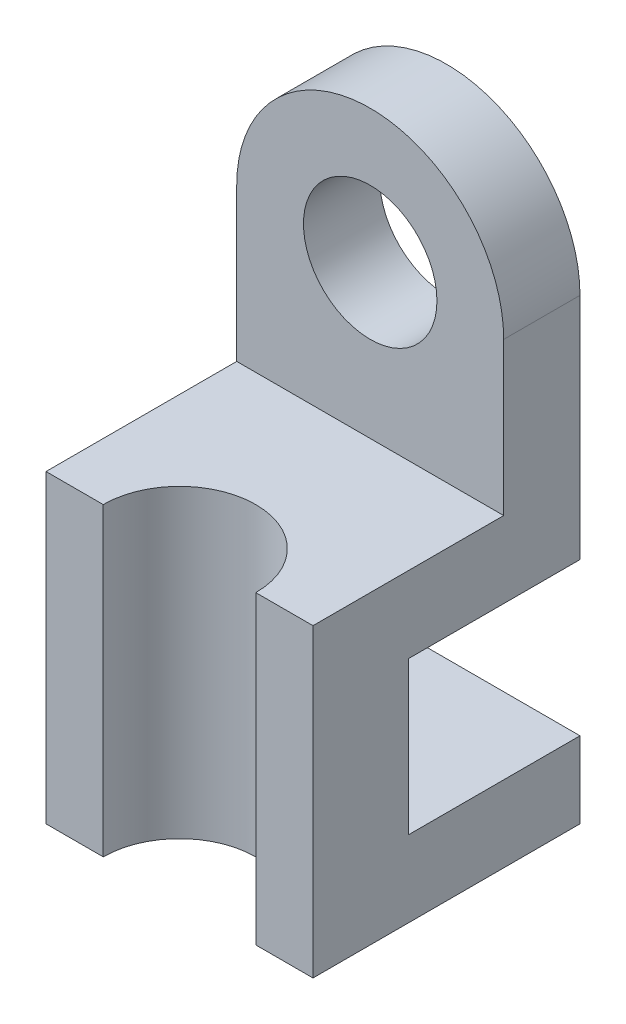
ISO-10303-21;
HEADER;
FILE_DESCRIPTION(('STEP AP214'),'2;1');
FILE_NAME('part.step','',(''),(''),'','','');
FILE_SCHEMA(('AUTOMOTIVE_DESIGN { 1 0 10303 214 1 1 1 1 }'));
ENDSEC;
DATA;
#1=APPLICATION_CONTEXT('core data for automotive mechanical design processes');
#2=APPLICATION_PROTOCOL_DEFINITION('international standard','automotive_design',2000,#1);
#3=PRODUCT_CONTEXT('',#1,'mechanical');
#4=PRODUCT('Part','Part','',(#3));
#5=PRODUCT_RELATED_PRODUCT_CATEGORY('part','',(#4));
#6=PRODUCT_DEFINITION_FORMATION('','',#4);
#7=PRODUCT_DEFINITION_CONTEXT('part definition',#1,'design');
#8=PRODUCT_DEFINITION('design','',#6,#7);
#9=PRODUCT_DEFINITION_SHAPE('','',#8);
#10=(LENGTH_UNIT() NAMED_UNIT(*) SI_UNIT(.MILLI.,.METRE.));
#11=(NAMED_UNIT(*) PLANE_ANGLE_UNIT() SI_UNIT($,.RADIAN.));
#12=(NAMED_UNIT(*) SI_UNIT($,.STERADIAN.) SOLID_ANGLE_UNIT());
#13=UNCERTAINTY_MEASURE_WITH_UNIT(LENGTH_MEASURE(1.E-05),#10,'distance_accuracy_value','');
#14=(GEOMETRIC_REPRESENTATION_CONTEXT(3) GLOBAL_UNCERTAINTY_ASSIGNED_CONTEXT((#13)) GLOBAL_UNIT_ASSIGNED_CONTEXT((#10,
#11,#12)) REPRESENTATION_CONTEXT('',''));
#15=CARTESIAN_POINT('',(0.,0.,0.));
#16=DIRECTION('',(0.,0.,1.));
#17=DIRECTION('',(1.,0.,0.));
#18=AXIS2_PLACEMENT_3D('',#15,#16,#17);
#19=CARTESIAN_POINT('',(-35.,20.,35.));
#20=DIRECTION('',(0.,0.,-1.));
#21=DIRECTION('',(-1.,0.,0.));
#22=AXIS2_PLACEMENT_3D('',#19,#20,#21);
#23=PLANE('',#22);
#24=DIRECTION('',(1.,0.,0.));
#25=VECTOR('',#24,1.);
#26=CARTESIAN_POINT('',(-35.,0.,35.));
#27=LINE('',#26,#25);
#28=CARTESIAN_POINT('',(-35.,0.,35.));
#29=VERTEX_POINT('',#28);
#30=CARTESIAN_POINT('',(-20.,0.,35.));
#31=VERTEX_POINT('',#30);
#32=EDGE_CURVE('E141',#29,#31,#27,.T.);
#33=ORIENTED_EDGE('',*,*,#32,.T.);
#34=DIRECTION('',(0.,1.,0.));
#35=VECTOR('',#34,1.);
#36=CARTESIAN_POINT('',(-20.,-128.,35.));
#37=LINE('',#36,#35);
#38=CARTESIAN_POINT('',(-20.,80.,35.));
#39=VERTEX_POINT('',#38);
#40=EDGE_CURVE('E132',#31,#39,#37,.T.);
#41=ORIENTED_EDGE('',*,*,#40,.T.);
#42=DIRECTION('',(1.,0.,0.));
#43=VECTOR('',#42,1.);
#44=CARTESIAN_POINT('',(-35.,80.,35.));
#45=LINE('',#44,#43);
#46=CARTESIAN_POINT('',(-35.,80.,35.));
#47=VERTEX_POINT('',#46);
#48=EDGE_CURVE('E142',#47,#39,#45,.T.);
#49=ORIENTED_EDGE('',*,*,#48,.F.);
#50=DIRECTION('',(0.,-1.,0.));
#51=VECTOR('',#50,1.);
#52=CARTESIAN_POINT('',(-35.,20.,35.));
#53=LINE('',#52,#51);
#54=EDGE_CURVE('E199',#47,#29,#53,.T.);
#55=ORIENTED_EDGE('',*,*,#54,.T.);
#56=EDGE_LOOP('',(#33,#41,#49,#55));
#57=FACE_BOUND('',#56,.T.);
#58=ADVANCED_FACE('F43',(#57),#23,.F.);
#59=CARTESIAN_POINT('',(35.,20.,0.));
#60=DIRECTION('',(-1.,0.,0.));
#61=DIRECTION('',(0.,0.,1.));
#62=AXIS2_PLACEMENT_3D('',#59,#60,#61);
#63=PLANE('',#62);
#64=DIRECTION('',(0.,0.,-1.));
#65=VECTOR('',#64,1.);
#66=CARTESIAN_POINT('',(35.,0.,0.));
#67=LINE('',#66,#65);
#68=CARTESIAN_POINT('',(35.,0.,35.));
#69=VERTEX_POINT('',#68);
#70=CARTESIAN_POINT('',(35.,0.,-35.));
#71=VERTEX_POINT('',#70);
#72=EDGE_CURVE('E181',#69,#71,#67,.T.);
#73=ORIENTED_EDGE('',*,*,#72,.T.);
#74=DIRECTION('',(0.,-1.,0.));
#75=VECTOR('',#74,1.);
#76=CARTESIAN_POINT('',(35.,20.,-35.));
#77=LINE('',#76,#75);
#78=CARTESIAN_POINT('',(35.,20.,-35.));
#79=VERTEX_POINT('',#78);
#80=EDGE_CURVE('E11',#79,#71,#77,.T.);
#81=ORIENTED_EDGE('',*,*,#80,.F.);
#82=DIRECTION('',(0.,0.,-1.));
#83=VECTOR('',#82,1.);
#84=CARTESIAN_POINT('',(35.,20.,35.));
#85=LINE('',#84,#83);
#86=CARTESIAN_POINT('',(35.,20.,9.99999999999999));
#87=VERTEX_POINT('',#86);
#88=EDGE_CURVE('E185',#87,#79,#85,.T.);
#89=ORIENTED_EDGE('',*,*,#88,.F.);
#90=DIRECTION('',(0.,-1.,0.));
#91=VECTOR('',#90,1.);
#92=CARTESIAN_POINT('',(35.,60.,9.99999999999999));
#93=LINE('',#92,#91);
#94=CARTESIAN_POINT('',(35.,60.,9.99999999999999));
#95=VERTEX_POINT('',#94);
#96=EDGE_CURVE('E178',#95,#87,#93,.T.);
#97=ORIENTED_EDGE('',*,*,#96,.F.);
#98=DIRECTION('',(0.,0.,-1.));
#99=VECTOR('',#98,1.);
#100=CARTESIAN_POINT('',(35.,60.,35.));
#101=LINE('',#100,#99);
#102=CARTESIAN_POINT('',(35.,60.,-35.));
#103=VERTEX_POINT('',#102);
#104=EDGE_CURVE('E157',#95,#103,#101,.T.);
#105=ORIENTED_EDGE('',*,*,#104,.T.);
#106=DIRECTION('',(0.,-1.,0.));
#107=VECTOR('',#106,1.);
#108=CARTESIAN_POINT('',(35.,80.,-35.));
#109=LINE('',#108,#107);
#110=CARTESIAN_POINT('',(35.,120.,-35.));
#111=VERTEX_POINT('',#110);
#112=EDGE_CURVE('E168',#111,#103,#109,.T.);
#113=ORIENTED_EDGE('',*,*,#112,.F.);
#114=DIRECTION('',(0.,0.,-1.));
#115=VECTOR('',#114,1.);
#116=CARTESIAN_POINT('',(35.,120.,-35.));
#117=LINE('',#116,#115);
#118=CARTESIAN_POINT('',(35.,120.,-15.));
#119=VERTEX_POINT('',#118);
#120=EDGE_CURVE('E233',#119,#111,#117,.T.);
#121=ORIENTED_EDGE('',*,*,#120,.F.);
#122=DIRECTION('',(0.,-1.,0.));
#123=VECTOR('',#122,1.);
#124=CARTESIAN_POINT('',(35.,120.,-15.));
#125=LINE('',#124,#123);
#126=CARTESIAN_POINT('',(35.,80.,-15.));
#127=VERTEX_POINT('',#126);
#128=EDGE_CURVE('E234',#119,#127,#125,.T.);
#129=ORIENTED_EDGE('',*,*,#128,.T.);
#130=DIRECTION('',(0.,0.,-1.));
#131=VECTOR('',#130,1.);
#132=CARTESIAN_POINT('',(35.,80.,35.));
#133=LINE('',#132,#131);
#134=CARTESIAN_POINT('',(35.,80.,35.));
#135=VERTEX_POINT('',#134);
#136=EDGE_CURVE('E149',#135,#127,#133,.T.);
#137=ORIENTED_EDGE('',*,*,#136,.F.);
#138=DIRECTION('',(0.,-1.,0.));
#139=VECTOR('',#138,1.);
#140=CARTESIAN_POINT('',(35.,20.,35.));
#141=LINE('',#140,#139);
#142=EDGE_CURVE('E189',#135,#69,#141,.T.);
#143=ORIENTED_EDGE('',*,*,#142,.T.);
#144=EDGE_LOOP('',(#73,#81,#89,#97,#105,#113,#121,#129,#137,#143));
#145=FACE_BOUND('',#144,.T.);
#146=ADVANCED_FACE('F44',(#145),#63,.F.);
#147=CARTESIAN_POINT('',(35.,20.,-35.));
#148=DIRECTION('',(0.,0.,1.));
#149=DIRECTION('',(1.,0.,0.));
#150=AXIS2_PLACEMENT_3D('',#147,#148,#149);
#151=PLANE('',#150);
#152=DIRECTION('',(-1.,0.,0.));
#153=VECTOR('',#152,1.);
#154=CARTESIAN_POINT('',(35.,0.,-35.));
#155=LINE('',#154,#153);
#156=CARTESIAN_POINT('',(-35.,0.,-35.));
#157=VERTEX_POINT('',#156);
#158=EDGE_CURVE('E188',#71,#157,#155,.T.);
#159=ORIENTED_EDGE('',*,*,#158,.T.);
#160=DIRECTION('',(0.,-1.,0.));
#161=VECTOR('',#160,1.);
#162=CARTESIAN_POINT('',(-35.,20.,-35.));
#163=LINE('',#162,#161);
#164=CARTESIAN_POINT('',(-35.,20.,-35.));
#165=VERTEX_POINT('',#164);
#166=EDGE_CURVE('E51',#165,#157,#163,.T.);
#167=ORIENTED_EDGE('',*,*,#166,.F.);
#168=DIRECTION('',(-1.,0.,0.));
#169=VECTOR('',#168,1.);
#170=CARTESIAN_POINT('',(35.,20.,-35.));
#171=LINE('',#170,#169);
#172=EDGE_CURVE('E183',#79,#165,#171,.T.);
#173=ORIENTED_EDGE('',*,*,#172,.F.);
#174=ORIENTED_EDGE('',*,*,#80,.T.);
#175=EDGE_LOOP('',(#159,#167,#173,#174));
#176=FACE_BOUND('',#175,.T.);
#177=ADVANCED_FACE('F261',(#176),#151,.F.);
#178=CARTESIAN_POINT('',(-35.,20.,-35.));
#179=DIRECTION('',(1.,0.,0.));
#180=DIRECTION('',(0.,0.,-1.));
#181=AXIS2_PLACEMENT_3D('',#178,#179,#180);
#182=PLANE('',#181);
#183=DIRECTION('',(0.,0.,1.));
#184=VECTOR('',#183,1.);
#185=CARTESIAN_POINT('',(-35.,0.,-35.));
#186=LINE('',#185,#184);
#187=EDGE_CURVE('E195',#157,#29,#186,.T.);
#188=ORIENTED_EDGE('',*,*,#187,.T.);
#189=ORIENTED_EDGE('',*,*,#54,.F.);
#190=DIRECTION('',(0.,0.,1.));
#191=VECTOR('',#190,1.);
#192=CARTESIAN_POINT('',(-35.,80.,-35.));
#193=LINE('',#192,#191);
#194=CARTESIAN_POINT('',(-35.,80.,-15.));
#195=VERTEX_POINT('',#194);
#196=EDGE_CURVE('E147',#195,#47,#193,.T.);
#197=ORIENTED_EDGE('',*,*,#196,.F.);
#198=DIRECTION('',(0.,-1.,0.));
#199=VECTOR('',#198,1.);
#200=CARTESIAN_POINT('',(-35.,120.,-15.));
#201=LINE('',#200,#199);
#202=CARTESIAN_POINT('',(-35.,120.,-15.));
#203=VERTEX_POINT('',#202);
#204=EDGE_CURVE('E159',#203,#195,#201,.T.);
#205=ORIENTED_EDGE('',*,*,#204,.F.);
#206=DIRECTION('',(0.,0.,1.));
#207=VECTOR('',#206,1.);
#208=CARTESIAN_POINT('',(-35.,120.,-15.));
#209=LINE('',#208,#207);
#210=CARTESIAN_POINT('',(-35.,120.,-35.));
#211=VERTEX_POINT('',#210);
#212=EDGE_CURVE('E226',#211,#203,#209,.T.);
#213=ORIENTED_EDGE('',*,*,#212,.F.);
#214=DIRECTION('',(0.,-1.,0.));
#215=VECTOR('',#214,1.);
#216=CARTESIAN_POINT('',(-35.,80.,-35.));
#217=LINE('',#216,#215);
#218=CARTESIAN_POINT('',(-35.,60.,-35.));
#219=VERTEX_POINT('',#218);
#220=EDGE_CURVE('E151',#211,#219,#217,.T.);
#221=ORIENTED_EDGE('',*,*,#220,.T.);
#222=DIRECTION('',(0.,0.,1.));
#223=VECTOR('',#222,1.);
#224=CARTESIAN_POINT('',(-35.,60.,-35.));
#225=LINE('',#224,#223);
#226=CARTESIAN_POINT('',(-35.,60.,9.99999999999999));
#227=VERTEX_POINT('',#226);
#228=EDGE_CURVE('E156',#219,#227,#225,.T.);
#229=ORIENTED_EDGE('',*,*,#228,.T.);
#230=DIRECTION('',(0.,-1.,0.));
#231=VECTOR('',#230,1.);
#232=CARTESIAN_POINT('',(-35.,60.,9.99999999999999));
#233=LINE('',#232,#231);
#234=CARTESIAN_POINT('',(-35.,20.,9.99999999999999));
#235=VERTEX_POINT('',#234);
#236=EDGE_CURVE('E173',#227,#235,#233,.T.);
#237=ORIENTED_EDGE('',*,*,#236,.T.);
#238=DIRECTION('',(0.,0.,1.));
#239=VECTOR('',#238,1.);
#240=CARTESIAN_POINT('',(-35.,20.,-35.));
#241=LINE('',#240,#239);
#242=EDGE_CURVE('E187',#165,#235,#241,.T.);
#243=ORIENTED_EDGE('',*,*,#242,.F.);
#244=ORIENTED_EDGE('',*,*,#166,.T.);
#245=EDGE_LOOP('',(#188,#189,#197,#205,#213,#221,#229,#237,#243,#244));
#246=FACE_BOUND('',#245,.T.);
#247=ADVANCED_FACE('F202',(#246),#182,.F.);
#248=CARTESIAN_POINT('',(20.,80.,35.));
#249=VERTEX_POINT('',#248);
#250=EDGE_CURVE('E146',#249,#135,#45,.T.);
#251=ORIENTED_EDGE('',*,*,#250,.F.);
#252=DIRECTION('',(0.,1.,0.));
#253=VECTOR('',#252,1.);
#254=CARTESIAN_POINT('',(20.,-128.,35.));
#255=LINE('',#254,#253);
#256=CARTESIAN_POINT('',(20.,0.,35.));
#257=VERTEX_POINT('',#256);
#258=EDGE_CURVE('E59',#257,#249,#255,.T.);
#259=ORIENTED_EDGE('',*,*,#258,.F.);
#260=EDGE_CURVE('E191',#257,#69,#27,.T.);
#261=ORIENTED_EDGE('',*,*,#260,.T.);
#262=ORIENTED_EDGE('',*,*,#142,.F.);
#263=EDGE_LOOP('',(#251,#259,#261,#262));
#264=FACE_BOUND('',#263,.T.);
#265=ADVANCED_FACE('F270',(#264),#23,.F.);
#266=CARTESIAN_POINT('',(0.,20.,0.));
#267=DIRECTION('',(0.,1.,0.));
#268=DIRECTION('',(0.,0.,1.));
#269=AXIS2_PLACEMENT_3D('',#266,#267,#268);
#270=PLANE('',#269);
#271=DIRECTION('',(-1.,0.,0.));
#272=VECTOR('',#271,1.);
#273=CARTESIAN_POINT('',(0.,20.,9.99999999999999));
#274=LINE('',#273,#272);
#275=EDGE_CURVE('E169',#87,#235,#274,.T.);
#276=ORIENTED_EDGE('',*,*,#275,.F.);
#277=ORIENTED_EDGE('',*,*,#88,.T.);
#278=ORIENTED_EDGE('',*,*,#172,.T.);
#279=ORIENTED_EDGE('',*,*,#242,.T.);
#280=EDGE_LOOP('',(#276,#277,#278,#279));
#281=FACE_BOUND('',#280,.T.);
#282=ADVANCED_FACE('F258',(#281),#270,.T.);
#283=CARTESIAN_POINT('',(0.,0.,0.));
#284=DIRECTION('',(0.,1.,0.));
#285=DIRECTION('',(0.,0.,1.));
#286=AXIS2_PLACEMENT_3D('',#283,#284,#285);
#287=PLANE('',#286);
#288=ORIENTED_EDGE('',*,*,#260,.F.);
#289=CARTESIAN_POINT('',(0.,0.,35.));
#290=DIRECTION('',(0.,1.,0.));
#291=DIRECTION('',(0.,0.,1.));
#292=AXIS2_PLACEMENT_3D('',#289,#290,#291);
#293=CIRCLE('',#292,20.);
#294=EDGE_CURVE('E215',#257,#31,#293,.T.);
#295=ORIENTED_EDGE('',*,*,#294,.T.);
#296=ORIENTED_EDGE('',*,*,#32,.F.);
#297=ORIENTED_EDGE('',*,*,#187,.F.);
#298=ORIENTED_EDGE('',*,*,#158,.F.);
#299=ORIENTED_EDGE('',*,*,#72,.F.);
#300=EDGE_LOOP('',(#288,#295,#296,#297,#298,#299));
#301=FACE_BOUND('',#300,.T.);
#302=ADVANCED_FACE('F208',(#301),#287,.F.);
#303=CARTESIAN_POINT('',(0.,60.,9.99999999999999));
#304=DIRECTION('',(0.,0.,1.));
#305=DIRECTION('',(1.,0.,0.));
#306=AXIS2_PLACEMENT_3D('',#303,#304,#305);
#307=PLANE('',#306);
#308=ORIENTED_EDGE('',*,*,#275,.T.);
#309=ORIENTED_EDGE('',*,*,#236,.F.);
#310=DIRECTION('',(-1.,0.,0.));
#311=VECTOR('',#310,1.);
#312=CARTESIAN_POINT('',(0.,60.,9.99999999999999));
#313=LINE('',#312,#311);
#314=EDGE_CURVE('E167',#95,#227,#313,.T.);
#315=ORIENTED_EDGE('',*,*,#314,.F.);
#316=ORIENTED_EDGE('',*,*,#96,.T.);
#317=EDGE_LOOP('',(#308,#309,#315,#316));
#318=FACE_BOUND('',#317,.T.);
#319=ADVANCED_FACE('F253',(#318),#307,.F.);
#320=CARTESIAN_POINT('',(0.,60.,0.));
#321=DIRECTION('',(0.,1.,0.));
#322=DIRECTION('',(0.,0.,1.));
#323=AXIS2_PLACEMENT_3D('',#320,#321,#322);
#324=PLANE('',#323);
#325=ORIENTED_EDGE('',*,*,#104,.F.);
#326=ORIENTED_EDGE('',*,*,#314,.T.);
#327=ORIENTED_EDGE('',*,*,#228,.F.);
#328=DIRECTION('',(-1.,0.,0.));
#329=VECTOR('',#328,1.);
#330=CARTESIAN_POINT('',(35.,60.,-35.));
#331=LINE('',#330,#329);
#332=EDGE_CURVE('E162',#103,#219,#331,.T.);
#333=ORIENTED_EDGE('',*,*,#332,.F.);
#334=EDGE_LOOP('',(#325,#326,#327,#333));
#335=FACE_BOUND('',#334,.T.);
#336=ADVANCED_FACE('F255',(#335),#324,.F.);
#337=CARTESIAN_POINT('',(35.,80.,-35.));
#338=DIRECTION('',(0.,0.,1.));
#339=DIRECTION('',(1.,0.,0.));
#340=AXIS2_PLACEMENT_3D('',#337,#338,#339);
#341=PLANE('',#340);
#342=CARTESIAN_POINT('',(0.,120.,-35.));
#343=DIRECTION('',(0.,0.,1.));
#344=DIRECTION('',(1.,0.,0.));
#345=AXIS2_PLACEMENT_3D('',#342,#343,#344);
#346=CIRCLE('',#345,17.5);
#347=CARTESIAN_POINT('',(17.5,120.,-35.));
#348=VERTEX_POINT('',#347);
#349=EDGE_CURVE('E216',#348,#348,#346,.T.);
#350=ORIENTED_EDGE('',*,*,#349,.T.);
#351=EDGE_LOOP('',(#350));
#352=FACE_BOUND('',#351,.T.);
#353=ORIENTED_EDGE('',*,*,#332,.T.);
#354=ORIENTED_EDGE('',*,*,#220,.F.);
#355=CARTESIAN_POINT('',(0.,120.,-35.));
#356=DIRECTION('',(0.,0.,1.));
#357=DIRECTION('',(1.,0.,0.));
#358=AXIS2_PLACEMENT_3D('',#355,#356,#357);
#359=CIRCLE('',#358,35.);
#360=EDGE_CURVE('E223',#111,#211,#359,.T.);
#361=ORIENTED_EDGE('',*,*,#360,.F.);
#362=ORIENTED_EDGE('',*,*,#112,.T.);
#363=EDGE_LOOP('',(#353,#354,#361,#362));
#364=FACE_BOUND('',#363,.T.);
#365=ADVANCED_FACE('F250',(#352,#364),#341,.F.);
#366=CARTESIAN_POINT('',(0.,80.,0.));
#367=DIRECTION('',(0.,1.,0.));
#368=DIRECTION('',(0.,0.,1.));
#369=AXIS2_PLACEMENT_3D('',#366,#367,#368);
#370=PLANE('',#369);
#371=CARTESIAN_POINT('',(0.,80.,35.));
#372=DIRECTION('',(0.,1.,0.));
#373=DIRECTION('',(0.,0.,1.));
#374=AXIS2_PLACEMENT_3D('',#371,#372,#373);
#375=CIRCLE('',#374,20.);
#376=EDGE_CURVE('E126',#249,#39,#375,.T.);
#377=ORIENTED_EDGE('',*,*,#376,.F.);
#378=ORIENTED_EDGE('',*,*,#250,.T.);
#379=ORIENTED_EDGE('',*,*,#136,.T.);
#380=DIRECTION('',(1.,0.,0.));
#381=VECTOR('',#380,1.);
#382=CARTESIAN_POINT('',(35.,80.,-15.));
#383=LINE('',#382,#381);
#384=EDGE_CURVE('E66',#195,#127,#383,.T.);
#385=ORIENTED_EDGE('',*,*,#384,.F.);
#386=ORIENTED_EDGE('',*,*,#196,.T.);
#387=ORIENTED_EDGE('',*,*,#48,.T.);
#388=EDGE_LOOP('',(#377,#378,#379,#385,#386,#387));
#389=FACE_BOUND('',#388,.T.);
#390=ADVANCED_FACE('F143',(#389),#370,.T.);
#391=CARTESIAN_POINT('',(35.,120.,-15.));
#392=DIRECTION('',(0.,0.,-1.));
#393=DIRECTION('',(-1.,0.,0.));
#394=AXIS2_PLACEMENT_3D('',#391,#392,#393);
#395=PLANE('',#394);
#396=CARTESIAN_POINT('',(0.,120.,-15.));
#397=DIRECTION('',(0.,0.,1.));
#398=DIRECTION('',(1.,0.,0.));
#399=AXIS2_PLACEMENT_3D('',#396,#397,#398);
#400=CIRCLE('',#399,17.5);
#401=CARTESIAN_POINT('',(17.5,120.,-15.));
#402=VERTEX_POINT('',#401);
#403=EDGE_CURVE('E214',#402,#402,#400,.T.);
#404=ORIENTED_EDGE('',*,*,#403,.F.);
#405=EDGE_LOOP('',(#404));
#406=FACE_BOUND('',#405,.T.);
#407=ORIENTED_EDGE('',*,*,#384,.T.);
#408=ORIENTED_EDGE('',*,*,#128,.F.);
#409=CARTESIAN_POINT('',(0.,120.,-15.));
#410=DIRECTION('',(0.,0.,1.));
#411=DIRECTION('',(1.,0.,0.));
#412=AXIS2_PLACEMENT_3D('',#409,#410,#411);
#413=CIRCLE('',#412,35.);
#414=EDGE_CURVE('E225',#119,#203,#413,.T.);
#415=ORIENTED_EDGE('',*,*,#414,.T.);
#416=ORIENTED_EDGE('',*,*,#204,.T.);
#417=EDGE_LOOP('',(#407,#408,#415,#416));
#418=FACE_BOUND('',#417,.T.);
#419=ADVANCED_FACE('F237',(#406,#418),#395,.F.);
#420=CARTESIAN_POINT('',(0.,120.,-35.));
#421=DIRECTION('',(0.,0.,1.));
#422=DIRECTION('',(1.,0.,0.));
#423=AXIS2_PLACEMENT_3D('',#420,#421,#422);
#424=CYLINDRICAL_SURFACE('',#423,35.);
#425=ORIENTED_EDGE('',*,*,#414,.F.);
#426=ORIENTED_EDGE('',*,*,#120,.T.);
#427=ORIENTED_EDGE('',*,*,#360,.T.);
#428=ORIENTED_EDGE('',*,*,#212,.T.);
#429=EDGE_LOOP('',(#425,#426,#427,#428));
#430=FACE_BOUND('',#429,.T.);
#431=ADVANCED_FACE('F242',(#430),#424,.T.);
#432=CARTESIAN_POINT('',(0.,120.,-223.));
#433=DIRECTION('',(0.,0.,1.));
#434=DIRECTION('',(1.,0.,0.));
#435=AXIS2_PLACEMENT_3D('',#432,#433,#434);
#436=CYLINDRICAL_SURFACE('',#435,17.5);
#437=ORIENTED_EDGE('',*,*,#403,.T.);
#438=EDGE_LOOP('',(#437));
#439=FACE_BOUND('',#438,.T.);
#440=ORIENTED_EDGE('',*,*,#349,.F.);
#441=EDGE_LOOP('',(#440));
#442=FACE_BOUND('',#441,.T.);
#443=ADVANCED_FACE('F301',(#439,#442),#436,.F.);
#444=CARTESIAN_POINT('',(0.,-128.,35.));
#445=DIRECTION('',(0.,1.,0.));
#446=DIRECTION('',(0.,0.,1.));
#447=AXIS2_PLACEMENT_3D('',#444,#445,#446);
#448=CYLINDRICAL_SURFACE('',#447,20.);
#449=ORIENTED_EDGE('',*,*,#258,.T.);
#450=ORIENTED_EDGE('',*,*,#376,.T.);
#451=ORIENTED_EDGE('',*,*,#40,.F.);
#452=ORIENTED_EDGE('',*,*,#294,.F.);
#453=EDGE_LOOP('',(#449,#450,#451,#452));
#454=FACE_BOUND('',#453,.T.);
#455=ADVANCED_FACE('F131',(#454),#448,.F.);
#456=CLOSED_SHELL('',(#58,#146,#177,#247,#265,#282,#302,#319,#336,#365,#390,#419,#431,#443,#455));
#457=MANIFOLD_SOLID_BREP('B2',#456);
#458=ADVANCED_BREP_SHAPE_REPRESENTATION('',(#18,#457),#14);
#459=SHAPE_DEFINITION_REPRESENTATION(#9,#458);
ENDSEC;
END-ISO-10303-21;
